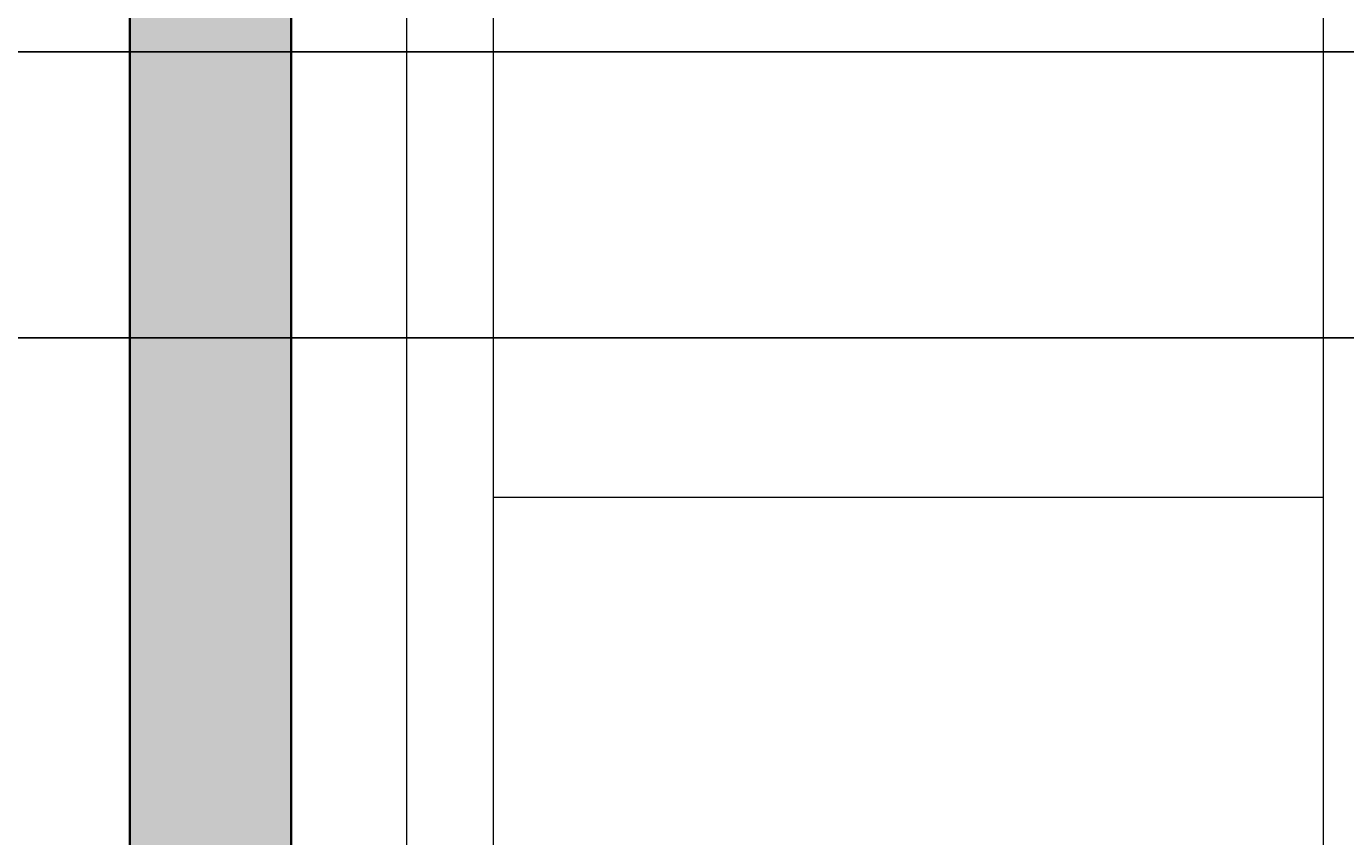
# Model space of a CAD drawing. Units: inches. Extents: x 1998 to 2588, y 1139 to 1977.
# Tile 44 of 134: x 2220 to 2257, y 1615 to 1637. Entities that reach past the tile are written whole.
import ezdxf

# ---------------------------------------------------------------- set-up
doc = ezdxf.new("R2010")
doc.units = ezdxf.units.IN
for name, color, linetype, lineweight in [('A-ANNO-DIMS', 2, 'Continuous', 18), ('A-WALL-PATT', 252, 'Continuous', 13), ('FUR', 21, 'Continuous', 18), ('WALL', 200, 'Continuous', 35)]:
    doc.layers.add(name, color=color, linetype=linetype, lineweight=lineweight)
doc.styles.get("Standard").update_dxf_attribs({"font": 'arial.ttf'})
doc.dimstyles.get("Standard").update_dxf_attribs({"dimtxt": 0.18, "dimasz": 0.18, "dimexe": 0.18, "dimexo": 0.0625, "dimgap": 0.09, "dimtad": 0, "dimtih": 1, "dimtoh": 1, "dimdec": 4, "dimzin": 0, "dimdsep": 46, "dimtxsty": 'Standard', "dimcen": 0.09, "dimadec": 0, "dimazin": 0, "dimtfac": 1, "dimtdec": 4, "dimtofl": 0, "dimtmove": 0, "dimatfit": 3, "dimfxl": 1, "dimtolj": 1, "dimtzin": 0, "dimarcsym": 0})

# ---------------------------------------------------------------- blocks, each defined once
blk = doc.blocks.new('SOFA-THREE-SEAT')
for p, q in [((47.077, 25.615), (47.077, 2.416)), ((0, 0), (74.336, 0))]:
    blk.add_line(p, q)
blk.add_lwpolyline([(3.604, 2.416), (71.008, 2.416), (71.008, 25.615), (3.604, 25.615)], close=True)
blk = doc.blocks.new('*D11')
at = {"layer": 'A-ANNO-DIMS', "color": 0, "lineweight": -2, "transparency": 16777216}
for p, q in [((2256.378, 1671.356), (2267.646, 1671.356)), ((2267.466, 1671.176), (2267.466, 1634.372)), ((2267.466, 1597.201), (2267.466, 1634.005)), ((2256.378, 1597.021), (2267.646, 1597.021))]:
    blk.add_line(p, q, dxfattribs=at)
at = {"layer": 'A-ANNO-DIMS', "color": 0, "transparency": 16777216}
for points in [[(2267.436, 1671.176), (2267.496, 1671.176), (2267.466, 1671.356)], [(2267.436, 1597.201), (2267.496, 1597.201), (2267.466, 1597.021)]]:
    blk.add_solid(points, dxfattribs=at)
at = {"layer": 'Defpoints', "color": 0, "transparency": 16777216}
for p in [(2256.316, 1671.356), (2256.316, 1597.021), (2267.466, 1597.021)]:
    blk.add_point(p, dxfattribs=at)
at = {"layer": 'A-ANNO-DIMS', "color": 0, "transparency": 16777216, "insert": (2267.466, 1634.189), "char_height": 0.18, "attachment_point": 5}
blk.add_mtext('\\A1;SOFA 74 TYP.', dxfattribs=at)
blk = doc.blocks.new('*D30')
at = {"layer": 'A-ANNO-DIMS', "color": 0, "lineweight": -2, "transparency": 16777216}
for p, q in [((2407.91, 1636.732), (1997.843, 1636.732)), ((1998.023, 1636.552), (1998.023, 1615.913)), ((1998.023, 1594.912), (1998.023, 1615.552)), ((2407.91, 1594.732), (1997.843, 1594.732))]:
    blk.add_line(p, q, dxfattribs=at)
at = {"layer": 'A-ANNO-DIMS', "color": 0, "transparency": 16777216}
for points in [[(1997.993, 1636.552), (1998.053, 1636.552), (1998.023, 1636.732)], [(1997.993, 1594.912), (1998.053, 1594.912), (1998.023, 1594.732)]]:
    blk.add_solid(points, dxfattribs=at)
at = {"layer": 'Defpoints', "color": 0, "transparency": 16777216}
for p in [(1998.023, 1636.732), (2407.973, 1636.732), (2407.973, 1594.732)]:
    blk.add_point(p, dxfattribs=at)
at = {"layer": 'A-ANNO-DIMS', "color": 0, "transparency": 16777216, "insert": (1998.023, 1615.732), "char_height": 0.18, "attachment_point": 5}
blk.add_mtext('\\A1;42', dxfattribs=at)
blk = doc.blocks.new('*D39')
at = {"layer": 'A-ANNO-DIMS', "color": 0, "lineweight": -2, "transparency": 16777216}
for p, q in [((2115.035, 1628.742), (2588.309, 1628.742)), ((2588.129, 1628.562), (2588.129, 1612.685)), ((2588.129, 1596.444), (2588.129, 1612.321)), ((2115.035, 1596.264), (2588.309, 1596.264))]:
    blk.add_line(p, q, dxfattribs=at)
at = {"layer": 'A-ANNO-DIMS', "color": 0, "transparency": 16777216}
for points in [[(2588.099, 1628.562), (2588.159, 1628.562), (2588.129, 1628.742)], [(2588.099, 1596.444), (2588.159, 1596.444), (2588.129, 1596.264)]]:
    blk.add_solid(points, dxfattribs=at)
at = {"layer": 'Defpoints', "color": 0, "transparency": 16777216}
for p in [(2114.973, 1628.742), (2588.129, 1628.742), (2114.973, 1596.264)]:
    blk.add_point(p, dxfattribs=at)
at = {"layer": 'A-ANNO-DIMS', "color": 0, "transparency": 16777216, "insert": (2588.129, 1612.503), "char_height": 0.18, "attachment_point": 5}
blk.add_mtext('\\A1;32.48', dxfattribs=at)

msp = doc.modelspace()

# ---------------------------------------------------------------- hatches: boundary and pattern name
at = {"layer": 'A-WALL-PATT'}
h = msp.add_hatch(color=256, dxfattribs=at)
h.dxf.hatch_style = 1
h.paths.add_polyline_path([(2527.4729, 1362.2324), (2510.9729, 1362.2324), (2510.9729, 1357.7324), (2518.4729, 1357.7324), (2518.4729, 1237.7324), (2503.1458, 1237.7324), (2503.1458, 1228.7324), (2527.4729, 1228.7324)])
h.paths.add_polyline_path([(2490.5682, 1362.2324), (2398.4729, 1362.2324), (2398.4729, 1357.7324), (2490.5682, 1357.7324)])
h.paths.add_polyline_path([(2224.9729, 1264.7324), (2222.9729, 1264.7324), (2222.9729, 1232.4125), (2341.4729, 1232.4125), (2341.4729, 1234.4125), (2224.9729, 1234.4125)])
h.paths.add_polyline_path([(2334.5332, 1273.7324), (2264.7638, 1273.7324), (2264.7638, 1269.5611, -0.043659), (2264.3413, 1264.7324), (2334.5332, 1264.7324)])
h.paths.add_polyline_path([(2236.9551, 1273.7324), (2234.4125, 1273.7324), (2234.4125, 1264.7324), (2236.9551, 1264.7324), (2236.9551, 1269.5611)])
h.paths.add_polyline_path([(2222.9729, 1293.2324), (2096.9729, 1293.2324), (2096.9729, 1345.0966), (2087.9729, 1345.0966), (2087.9729, 1284.2324), (2222.9729, 1284.2324), (2222.9729, 1285.137)])
h.paths.add_polyline_path([(2096.9729, 1458.7927), (2087.9729, 1458.7927), (2087.9729, 1417.7324), (2087.9729, 1413.2324), (2096.9729, 1413.2324), (2096.9729, 1417.7324)])
h.paths.add_polyline_path([(2096.9729, 1413.2324), (2087.9729, 1413.2324), (2087.9729, 1365.5012), (2096.9729, 1365.5012), (2096.9729, 1369.3358)])
h.paths.add_polyline_path([(2186.2943, 1417.7324), (2138.6074, 1417.7324), (2096.9729, 1417.7324), (2096.9729, 1413.2324), (2138.6074, 1413.2324), (2186.2943, 1413.2324)])
h.paths.add_polyline_path([(2181.4729, 1465.7324), (2176.9729, 1465.7324), (2176.9729, 1451.6434), (2181.4729, 1451.6434)])
h.paths.add_polyline_path([(2181.4729, 1422.1664), (2176.9729, 1422.1664), (2176.9729, 1417.7324), (2181.4729, 1417.7324)])
h.paths.add_polyline_path([(2063.9729, 1465.7324), (2087.9729, 1465.7324), (2087.9729, 1470.2324), (2059.4729, 1470.2324), (2059.4729, 1413.2324), (2087.9729, 1413.2324), (2087.9729, 1417.7324), (2063.9729, 1417.7324)])
h.paths.add_polyline_path([(2181.4729, 1755.2324), (2176.9729, 1755.2324), (2176.9729, 1748.6798), (2177.0513, 1748.6798), (2181.4729, 1748.6798)])
h.paths.add_polyline_path([(2227.4729, 1707.2324), (2220.4647, 1707.2324), (2220.4647, 1702.7324), (2222.9729, 1702.7324), (2222.9729, 1604.637), (2227.4729, 1604.637)])
h.paths.add_polyline_path([(2114.9729, 1702.7324), (2105.9729, 1702.7324), (2105.9729, 1628.4781, -0.0318759), (2110.1012, 1628.7416), (2114.9729, 1628.7416)])
h.paths.add_polyline_path([(2345.9729, 1739.3278), (2341.4729, 1739.3278), (2341.4729, 1647.5211), (2345.9729, 1647.5211)])
h.paths.add_polyline_path([(2350.6273, 1641.2324), (2345.9729, 1641.2324), (2345.9729, 1636.7324), (2350.6273, 1636.7324), (2350.6273, 1639.8729)])
h.paths.add_polyline_path([(2501.9729, 1641.2324), (2407.9729, 1641.2324), (2392.5005, 1641.2324), (2392.5005, 1639.8729), (2392.5005, 1636.7324), (2501.9729, 1636.7324)])
h.paths.add_polyline_path([(2510.9729, 1755.2324), (2501.9729, 1755.2324), (2501.9729, 1641.2324), (2510.9729, 1641.2324)])
h.paths.add_polyline_path([(2549.1786, 1641.2324), (2522.3775, 1641.2324), (2522.3775, 1636.7324), (2540.1786, 1636.7324), (2540.1786, 1480.7324), (2522.3775, 1480.7324), (2522.3775, 1476.2324), (2549.1786, 1476.2324)])
h.paths.add_polyline_path([(2498.1786, 1594.7324), (2407.9729, 1594.7324), (2407.9729, 1585.7324), (2416.9729, 1585.7324), (2489.1786, 1585.7324), (2489.1786, 1531.7324), (2416.9729, 1531.7324), (2407.9729, 1531.7324), (2407.9729, 1522.7324), (2498.1786, 1522.7324)])
h.paths.add_polyline_path([(2351.6437, 1480.7324), (2345.9729, 1480.7324), (2345.9729, 1476.2324), (2351.6437, 1476.2324), (2351.6437, 1477.5919)])
h.paths.add_polyline_path([(2501.9729, 1480.7324), (2498.1786, 1480.7324), (2407.9729, 1480.7324), (2393.5168, 1480.7324), (2393.5168, 1477.5919), (2393.5168, 1476.2324), (2501.9729, 1476.2324)])

# ---------------------------------------------------------------- linework, layer by layer
at = {"layer": 'WALL'}
for p, q in [((2227.4729, 1707.2324), (2227.4729, 1584.2324)), ((2222.9729, 1702.7324), (2222.9729, 1604.637))]:
    msp.add_line(p, q, dxfattribs=at)

# ---------------------------------------------------------------- block references
at = {"layer": 'FUR', "rotation": 270.0000000000001}
msp.add_blockref('SOFA-THREE-SEAT', (2230.701, 1671.3567), dxfattribs=at)

# ---------------------------------------------------------------- dimensions: what is measured, and where the dimension line sits
at = {"layer": 'A-ANNO-DIMS'}
dim = msp.add_linear_dim(base=(2267.4662, 1597.0205), p1=(2256.3158, 1671.3565), p2=(2256.3158, 1597.0205), angle=270, text='SOFA <> TYP.', dimstyle='Standard', override={"dimdec": 0, "dimlfac": 1, "dimrnd": 0, "dimzin": 0, "dimdsep": 46, "dimlunit": 2}, dxfattribs=at)
dim.commit()
dim.dimension.update_dxf_attribs({"geometry": '*D11', "text_midpoint": (2267.4662, 1634.1885)})
for base, p1, p2, override, picture, middle in [((1998.0229, 1636.7324), (2407.9729, 1594.7324), (2407.9729, 1636.7324), {"dimdec": 0, "dimlfac": 1, "dimrnd": 0, "dimzin": 0, "dimdsep": 46, "dimlunit": 2}, '*D30', (1998.0229, 1615.7324)), ((2588.1286, 1628.7416), (2114.9729, 1596.2642), (2114.9729, 1628.7416), {"dimdec": 2, "dimlfac": 1, "dimrnd": 0, "dimzin": 0, "dimdsep": 46, "dimlunit": 2}, '*D39', (2588.1286, 1612.5029))]:
    dim = msp.add_linear_dim(base=base, p1=p1, p2=p2, angle=90, dimstyle='Standard', override=override, dxfattribs=at)
    dim.commit()
    dim.dimension.update_dxf_attribs({"geometry": picture, "text_midpoint": middle})

doc.saveas('drawing.dxf')
